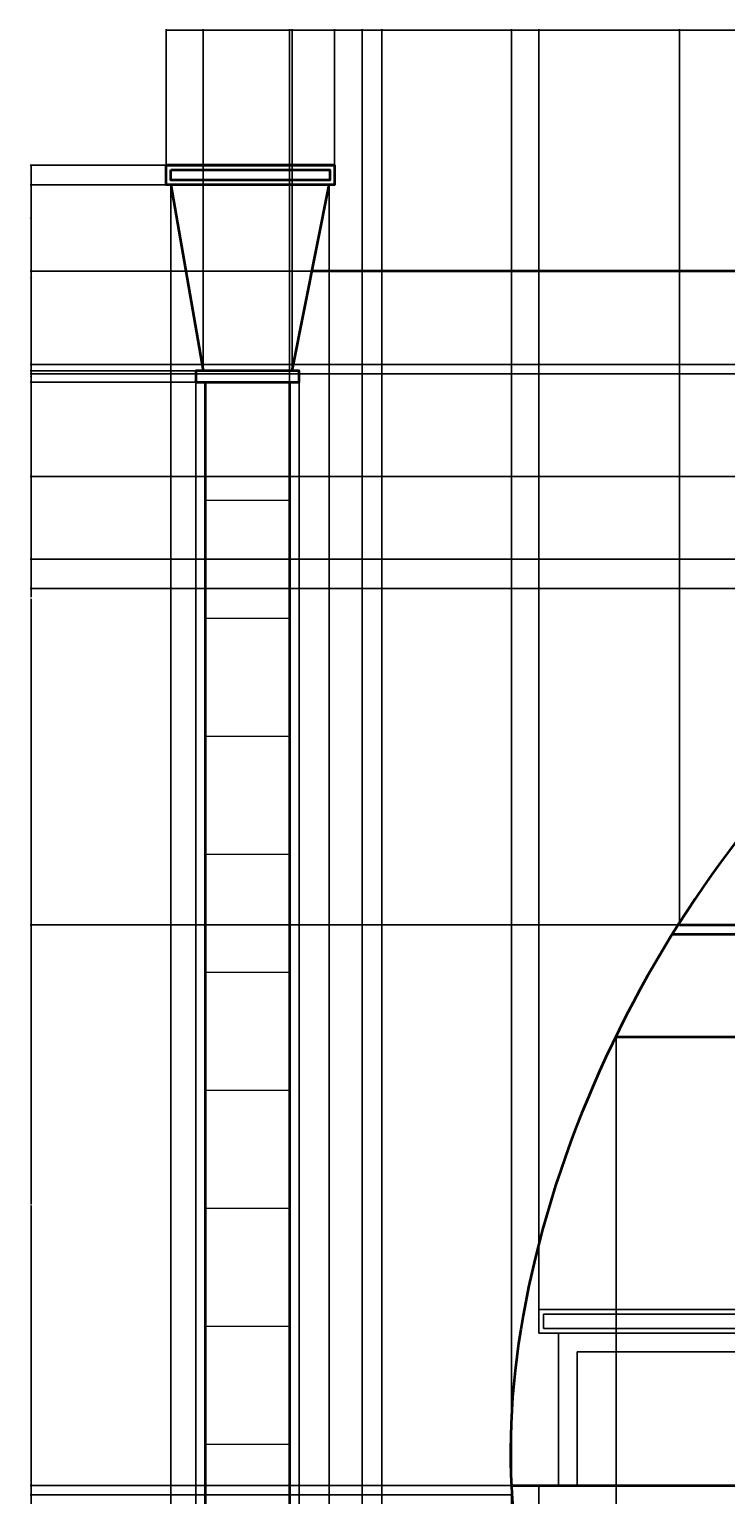
# Model space of a CAD drawing. Units: inches. Extents: x -19 to 408, y -26 to 603.
# Tile 5 of 7: x -19 to 130, y 289 to 603. Entities that reach past the tile are written whole.
import ezdxf

# ---------------------------------------------------------------- set-up
doc = ezdxf.new("R2010")
doc.units = ezdxf.units.IN
doc.header["$MEASUREMENT"] = 0
for name, color, linetype, lineweight in [('A-ANNO-DIMS', 2, 'Continuous', 18), ('A-ELEV', 7, 'Continuous', 35), ('A-GLAZ', 4, 'Continuous', 25), ('A-WALL-PATT', 8, 'Continuous', 13)]:
    doc.layers.add(name, color=color, linetype=linetype, lineweight=lineweight)
doc.styles.get("Standard").update_dxf_attribs({"font": 'arial.ttf'})
doc.dimstyles.get("Standard").update_dxf_attribs({"dimtxt": 0.18, "dimasz": 0.18, "dimexe": 0.18, "dimexo": 0.0625, "dimgap": 0.09, "dimtad": 0, "dimtih": 1, "dimtoh": 1, "dimdec": 4, "dimzin": 0, "dimdsep": 46, "dimtxsty": 'Standard', "dimcen": 0.09, "dimadec": 0, "dimazin": 0, "dimtfac": 1, "dimtdec": 4, "dimtofl": 0, "dimtmove": 0, "dimatfit": 3, "dimfxl": 1, "dimtolj": 1, "dimtzin": 0, "dimarcsym": 0})

# ---------------------------------------------------------------- blocks, each defined once
blk = doc.blocks.new('WIN-1200')
for points in [[(0, 32.56), (59.66, 32.56), (59.66, 37.64), (0, 37.64)], [(1, 33.56), (58.66, 33.56), (58.66, 36.64), (1, 36.64)]]:
    blk.add_lwpolyline(points, close=True)
for points in [[(4.17, 0), (4.17, 32.56), (55.99, 32.56), (55.99, 0)], [(8.17, 0), (8.17, 28.56), (51.99, 28.56), (51.99, 0)]]:
    blk.add_lwpolyline(points)
blk = doc.blocks.new('*D4')
at = {"layer": 'A-ANNO-DIMS', "color": 0, "lineweight": -2, "transparency": 16777216}
for p, q in [((89.99, 291.08), (89.99, 282.02)), ((149.65, 291.08), (149.65, 282.02)), ((90.17, 282.2), (118.7, 282.2)), ((149.47, 282.2), (120.94, 282.2))]:
    blk.add_line(p, q, dxfattribs=at)
at = {"layer": 'A-ANNO-DIMS', "color": 0, "transparency": 16777216}
for points in [[(90.17, 282.23), (90.17, 282.17), (89.99, 282.2)], [(149.47, 282.23), (149.47, 282.17), (149.65, 282.2)]]:
    blk.add_solid(points, dxfattribs=at)
at = {"layer": 'Defpoints', "color": 0, "transparency": 16777216}
for p in [(89.99, 291.15), (149.65, 291.15), (149.65, 282.2)]:
    blk.add_point(p, dxfattribs=at)
at = {"layer": 'A-ANNO-DIMS', "color": 0, "transparency": 16777216, "insert": (119.82, 282.2), "char_height": 0.18, "attachment_point": 5}
blk.add_mtext('\\A1;WINDOW 60 TYP.', dxfattribs=at)
blk = doc.blocks.new('*D15')
at = {"layer": 'A-ANNO-DIMS', "color": 0, "lineweight": -2, "transparency": 16777216}
for p, q in [((10.2, 573.88), (10.2, 602.9)), ((10.38, 602.72), (110.85, 602.72)), ((212.25, 602.72), (111.78, 602.72)), ((212.43, 551.17), (212.43, 602.9))]:
    blk.add_line(p, q, dxfattribs=at)
at = {"layer": 'A-ANNO-DIMS', "color": 0, "transparency": 16777216}
for points in [[(10.38, 602.75), (10.38, 602.69), (10.2, 602.72)], [(212.25, 602.75), (212.25, 602.69), (212.43, 602.72)]]:
    blk.add_solid(points, dxfattribs=at)
at = {"layer": 'Defpoints', "color": 0, "transparency": 16777216}
for p in [(212.43, 602.72), (10.2, 573.82), (212.43, 551.1)]:
    blk.add_point(p, dxfattribs=at)
at = {"layer": 'A-ANNO-DIMS', "color": 0, "transparency": 16777216, "insert": (111.32, 602.72), "char_height": 0.18, "attachment_point": 5}
blk.add_mtext('\\A1;202.23', dxfattribs=at)
blk = doc.blocks.new('*D19')
at = {"layer": 'A-ANNO-DIMS', "color": 0, "lineweight": -2, "transparency": 16777216}
for p, q in [((84.02, 291.15), (-18.88, 291.15)), ((-18.7, 290.97), (-18.7, 255.33)), ((-18.7, 219.33), (-18.7, 254.97)), ((36.51, 219.15), (-18.88, 219.15))]:
    blk.add_line(p, q, dxfattribs=at)
at = {"layer": 'A-ANNO-DIMS', "color": 0, "transparency": 16777216}
for points in [[(-18.73, 290.97), (-18.67, 290.97), (-18.7, 291.15)], [(-18.73, 219.33), (-18.67, 219.33), (-18.7, 219.15)]]:
    blk.add_solid(points, dxfattribs=at)
at = {"layer": 'Defpoints', "color": 0, "transparency": 16777216}
for p in [(-18.7, 291.15), (84.08, 291.15), (36.57, 219.15)]:
    blk.add_point(p, dxfattribs=at)
at = {"layer": 'A-ANNO-DIMS', "color": 0, "transparency": 16777216, "insert": (-18.7, 255.15), "char_height": 0.18, "attachment_point": 5}
blk.add_mtext('\\A1;72', dxfattribs=at)
blk = doc.blocks.new('*D20')
at = {"layer": 'A-ANNO-DIMS', "color": 0, "lineweight": -2, "transparency": 16777216}
for p, q in [((185.46, 411.15), (-18.88, 411.15)), ((-18.7, 410.97), (-18.7, 351.33)), ((-18.7, 291.33), (-18.7, 350.97)), ((84.02, 291.15), (-18.88, 291.15))]:
    blk.add_line(p, q, dxfattribs=at)
at = {"layer": 'A-ANNO-DIMS', "color": 0, "transparency": 16777216}
for points in [[(-18.73, 410.97), (-18.67, 410.97), (-18.7, 411.15)], [(-18.73, 291.33), (-18.67, 291.33), (-18.7, 291.15)]]:
    blk.add_solid(points, dxfattribs=at)
at = {"layer": 'Defpoints', "color": 0, "transparency": 16777216}
for p in [(-18.7, 411.15), (185.52, 411.15), (84.08, 291.15)]:
    blk.add_point(p, dxfattribs=at)
at = {"layer": 'A-ANNO-DIMS', "color": 0, "transparency": 16777216, "insert": (-18.7, 351.15), "char_height": 0.18, "attachment_point": 5}
blk.add_mtext('\\A1;120', dxfattribs=at)
blk = doc.blocks.new('*D21')
at = {"layer": 'A-ANNO-DIMS', "color": 0, "lineweight": -2, "transparency": 16777216}
for p, q in [((212.37, 551.1), (-18.88, 551.1)), ((-18.7, 550.92), (-18.7, 481.31)), ((-18.7, 411.33), (-18.7, 480.94)), ((185.46, 411.15), (-18.88, 411.15))]:
    blk.add_line(p, q, dxfattribs=at)
at = {"layer": 'A-ANNO-DIMS', "color": 0, "transparency": 16777216}
for points in [[(-18.73, 550.92), (-18.67, 550.92), (-18.7, 551.1)], [(-18.73, 411.33), (-18.67, 411.33), (-18.7, 411.15)]]:
    blk.add_solid(points, dxfattribs=at)
at = {"layer": 'Defpoints', "color": 0, "transparency": 16777216}
for p in [(-18.7, 551.1), (212.43, 551.1), (185.52, 411.15)]:
    blk.add_point(p, dxfattribs=at)
at = {"layer": 'A-ANNO-DIMS', "color": 0, "transparency": 16777216, "insert": (-18.7, 481.13), "char_height": 0.18, "attachment_point": 5}
blk.add_mtext('\\A1;139.96', dxfattribs=at)
blk = doc.blocks.new('*D22')
at = {"layer": 'A-ANNO-DIMS', "color": 0, "lineweight": -2, "transparency": 16777216}
for p, q in [((10.14, 573.82), (-18.88, 573.82)), ((-18.7, 573.64), (-18.7, 562.64)), ((-18.7, 551.28), (-18.7, 562.28)), ((212.37, 551.1), (-18.88, 551.1))]:
    blk.add_line(p, q, dxfattribs=at)
at = {"layer": 'A-ANNO-DIMS', "color": 0, "transparency": 16777216}
for points in [[(-18.73, 573.64), (-18.67, 573.64), (-18.7, 573.82)], [(-18.73, 551.28), (-18.67, 551.28), (-18.7, 551.1)]]:
    blk.add_solid(points, dxfattribs=at)
at = {"layer": 'Defpoints', "color": 0, "transparency": 16777216}
for p in [(-18.7, 573.82), (10.2, 573.82), (212.43, 551.1)]:
    blk.add_point(p, dxfattribs=at)
at = {"layer": 'A-ANNO-DIMS', "color": 0, "transparency": 16777216, "insert": (-18.7, 562.46), "char_height": 0.18, "attachment_point": 5}
blk.add_mtext('\\A1;22.714', dxfattribs=at)
blk = doc.blocks.new('*D28')
at = {"layer": 'A-ANNO-DIMS', "color": 0, "lineweight": -2, "transparency": 16777216}
for p, q in [((36.57, 300.05), (36.57, 602.9)), ((36.75, 602.72), (59.94, 602.72)), ((83.9, 602.72), (60.7, 602.72)), ((84.08, 291.21), (84.08, 602.9))]:
    blk.add_line(p, q, dxfattribs=at)
at = {"layer": 'A-ANNO-DIMS', "color": 0, "transparency": 16777216}
for points in [[(36.75, 602.75), (36.75, 602.69), (36.57, 602.72)], [(83.9, 602.75), (83.9, 602.69), (84.08, 602.72)]]:
    blk.add_solid(points, dxfattribs=at)
at = {"layer": 'Defpoints', "color": 0, "transparency": 16777216}
for p in [(84.08, 602.72), (36.57, 299.99), (84.08, 291.15)]:
    blk.add_point(p, dxfattribs=at)
at = {"layer": 'A-ANNO-DIMS', "color": 0, "transparency": 16777216, "insert": (60.32, 602.72), "char_height": 0.18, "attachment_point": 5}
blk.add_mtext('\\A1;47.51', dxfattribs=at)
blk = doc.blocks.new('*D35')
at = {"layer": 'A-ANNO-DIMS', "color": 0, "lineweight": -2, "transparency": 16777216}
for p, q in [((36.57, 171.21), (36.57, 602.9)), ((36.75, 602.72), (43.91, 602.72)), ((51.97, 602.72), (44.82, 602.72)), ((52.15, 203.77), (52.15, 602.9))]:
    blk.add_line(p, q, dxfattribs=at)
at = {"layer": 'A-ANNO-DIMS', "color": 0, "transparency": 16777216}
for points in [[(36.75, 602.75), (36.75, 602.69), (36.57, 602.72)], [(51.97, 602.75), (51.97, 602.69), (52.15, 602.72)]]:
    blk.add_solid(points, dxfattribs=at)
at = {"layer": 'Defpoints', "color": 0, "transparency": 16777216}
for p in [(52.15, 602.72), (52.15, 203.7), (36.57, 171.15)]:
    blk.add_point(p, dxfattribs=at)
at = {"layer": 'A-ANNO-DIMS', "color": 0, "transparency": 16777216, "insert": (44.36, 602.72), "char_height": 0.18, "attachment_point": 5}
blk.add_mtext('\\A1;15.582', dxfattribs=at)
blk = doc.blocks.new('*D36')
at = {"layer": 'A-ANNO-DIMS', "color": 0, "lineweight": -2, "transparency": 16777216}
for p, q in [((52.15, 203.77), (52.15, 602.9)), ((52.33, 602.72), (96.69, 602.72)), ((141.84, 602.72), (97.48, 602.72)), ((142.02, 171.21), (142.02, 602.9))]:
    blk.add_line(p, q, dxfattribs=at)
at = {"layer": 'A-ANNO-DIMS', "color": 0, "transparency": 16777216}
for points in [[(52.33, 602.75), (52.33, 602.69), (52.15, 602.72)], [(141.84, 602.75), (141.84, 602.69), (142.02, 602.72)]]:
    blk.add_solid(points, dxfattribs=at)
at = {"layer": 'Defpoints', "color": 0, "transparency": 16777216}
for p in [(142.02, 602.72), (52.15, 203.7), (142.02, 171.15)]:
    blk.add_point(p, dxfattribs=at)
at = {"layer": 'A-ANNO-DIMS', "color": 0, "transparency": 16777216, "insert": (97.09, 602.72), "char_height": 0.18, "attachment_point": 5}
blk.add_mtext('\\A1;89.87', dxfattribs=at)
blk = doc.blocks.new('*D45')
at = {"layer": 'A-ANNO-DIMS', "color": 0, "lineweight": -2, "transparency": 16777216}
for p, q in [((36.57, 219.21), (36.57, 602.9)), ((36.75, 602.72), (85.2, 602.72)), ((134.3, 602.72), (85.85, 602.72)), ((134.48, 220.21), (134.48, 602.9))]:
    blk.add_line(p, q, dxfattribs=at)
at = {"layer": 'A-ANNO-DIMS', "color": 0, "transparency": 16777216}
for points in [[(36.75, 602.75), (36.75, 602.69), (36.57, 602.72)], [(134.3, 602.75), (134.3, 602.69), (134.48, 602.72)]]:
    blk.add_solid(points, dxfattribs=at)
at = {"layer": 'Defpoints', "color": 0, "transparency": 16777216}
for p in [(134.48, 602.72), (134.48, 220.15), (36.57, 219.15)]:
    blk.add_point(p, dxfattribs=at)
at = {"layer": 'A-ANNO-DIMS', "color": 0, "transparency": 16777216, "insert": (85.52, 602.72), "char_height": 0.18, "attachment_point": 5}
blk.add_mtext('\\A1;97.9', dxfattribs=at)
blk = doc.blocks.new('*D47')
at = {"layer": 'A-ANNO-DIMS', "color": 0, "lineweight": -2, "transparency": 16777216}
for p, q in [((52.15, 203.77), (52.15, 602.9)), ((52.33, 602.72), (53.84, 602.72)), ((56.15, 602.72), (54.64, 602.72)), ((56.33, 203.77), (56.33, 602.9))]:
    blk.add_line(p, q, dxfattribs=at)
at = {"layer": 'A-ANNO-DIMS', "color": 0, "transparency": 16777216}
for points in [[(52.33, 602.75), (52.33, 602.69), (52.15, 602.72)], [(56.15, 602.75), (56.15, 602.69), (56.33, 602.72)]]:
    blk.add_solid(points, dxfattribs=at)
at = {"layer": 'Defpoints', "color": 0, "transparency": 16777216}
for p in [(56.33, 602.72), (52.15, 203.7), (56.33, 203.7)]:
    blk.add_point(p, dxfattribs=at)
at = {"layer": 'A-ANNO-DIMS', "color": 0, "transparency": 16777216, "insert": (54.24, 602.72), "char_height": 0.18, "attachment_point": 5}
blk.add_mtext('\\A1;4.173', dxfattribs=at)
blk = doc.blocks.new('*D60')
at = {"layer": 'A-ANNO-DIMS', "color": 0, "lineweight": -2, "transparency": 16777216}
for p, q in [((84.08, 291.08), (84.08, -25.93)), ((109.02, 267.08), (109.02, -25.93)), ((84.26, -25.75), (96.15, -25.75)), ((108.84, -25.75), (96.94, -25.75))]:
    blk.add_line(p, q, dxfattribs=at)
at = {"layer": 'A-ANNO-DIMS', "color": 0, "transparency": 16777216}
for points in [[(84.26, -25.72), (84.26, -25.78), (84.08, -25.75)], [(108.84, -25.72), (108.84, -25.78), (109.02, -25.75)]]:
    blk.add_solid(points, dxfattribs=at)
at = {"layer": 'Defpoints', "color": 0, "transparency": 16777216}
for p in [(84.08, 291.15), (109.02, 267.15), (109.02, -25.75)]:
    blk.add_point(p, dxfattribs=at)
at = {"layer": 'A-ANNO-DIMS', "color": 0, "transparency": 16777216, "insert": (96.55, -25.75), "char_height": 0.18, "attachment_point": 5}
blk.add_mtext('\\A1;24.94', dxfattribs=at)
blk = doc.blocks.new('*D66')
at = {"layer": 'A-ANNO-DIMS', "color": 0, "lineweight": -2, "transparency": 16777216}
for p, q in [((84.08, 291.21), (84.08, 602.9)), ((84.26, 602.72), (86.64, 602.72)), ((89.81, 602.72), (87.43, 602.72)), ((89.99, 323.77), (89.99, 602.9))]:
    blk.add_line(p, q, dxfattribs=at)
at = {"layer": 'A-ANNO-DIMS', "color": 0, "transparency": 16777216}
for points in [[(84.26, 602.75), (84.26, 602.69), (84.08, 602.72)], [(89.81, 602.75), (89.81, 602.69), (89.99, 602.72)]]:
    blk.add_solid(points, dxfattribs=at)
at = {"layer": 'Defpoints', "color": 0, "transparency": 16777216}
for p in [(89.99, 602.72), (89.99, 323.7), (84.08, 291.15)]:
    blk.add_point(p, dxfattribs=at)
at = {"layer": 'A-ANNO-DIMS', "color": 0, "transparency": 16777216, "insert": (87.03, 602.72), "char_height": 0.18, "attachment_point": 5}
blk.add_mtext('\\A1;5.912', dxfattribs=at)
blk = doc.blocks.new('*D68')
at = {"layer": 'A-ANNO-DIMS', "color": 0, "lineweight": -2, "transparency": 16777216}
for p, q in [((84.13, 289.15), (-18.88, 289.15)), ((-18.7, 288.97), (-18.7, 278.33)), ((-18.7, 267.33), (-18.7, 277.97)), ((87.66, 267.15), (-18.88, 267.15))]:
    blk.add_line(p, q, dxfattribs=at)
at = {"layer": 'A-ANNO-DIMS', "color": 0, "transparency": 16777216}
for points in [[(-18.73, 288.97), (-18.67, 288.97), (-18.7, 289.15)], [(-18.73, 267.33), (-18.67, 267.33), (-18.7, 267.15)]]:
    blk.add_solid(points, dxfattribs=at)
at = {"layer": 'Defpoints', "color": 0, "transparency": 16777216}
for p in [(-18.7, 289.15), (84.19, 289.15), (87.72, 267.15)]:
    blk.add_point(p, dxfattribs=at)
at = {"layer": 'A-ANNO-DIMS', "color": 0, "transparency": 16777216, "insert": (-18.7, 278.15), "char_height": 0.18, "attachment_point": 5}
blk.add_mtext('\\A1;22', dxfattribs=at)
blk = doc.blocks.new('*D69')
at = {"layer": 'A-ANNO-DIMS', "color": 0, "lineweight": -2, "transparency": 16777216}
for p, q in [((84.02, 291.15), (-18.88, 291.15)), ((84.13, 289.15), (-18.88, 289.15)), ((-18.7, 290.97), (-18.7, 290.33)), ((-18.7, 289.33), (-18.7, 289.97))]:
    blk.add_line(p, q, dxfattribs=at)
at = {"layer": 'A-ANNO-DIMS', "color": 0, "transparency": 16777216}
for points in [[(-18.73, 290.97), (-18.67, 290.97), (-18.7, 291.15)], [(-18.73, 289.33), (-18.67, 289.33), (-18.7, 289.15)]]:
    blk.add_solid(points, dxfattribs=at)
at = {"layer": 'Defpoints', "color": 0, "transparency": 16777216}
for p in [(-18.7, 291.15), (84.08, 291.15), (84.19, 289.15)]:
    blk.add_point(p, dxfattribs=at)
at = {"layer": 'A-ANNO-DIMS', "color": 0, "transparency": 16777216, "insert": (-18.7, 290.15), "char_height": 0.18, "attachment_point": 5}
blk.add_mtext('\\A1;2', dxfattribs=at)
blk = doc.blocks.new('*D79')
at = {"layer": 'A-ANNO-DIMS', "color": 0, "lineweight": -2, "transparency": 16777216}
for p, q in [((212.37, 489.45), (-18.88, 489.45)), ((-18.7, 489.27), (-18.7, 486.48)), ((-18.7, 483.33), (-18.7, 486.12)), ((212.37, 483.15), (-18.88, 483.15))]:
    blk.add_line(p, q, dxfattribs=at)
at = {"layer": 'A-ANNO-DIMS', "color": 0, "transparency": 16777216}
for points in [[(-18.73, 489.27), (-18.67, 489.27), (-18.7, 489.45)], [(-18.73, 483.33), (-18.67, 483.33), (-18.7, 483.15)]]:
    blk.add_solid(points, dxfattribs=at)
at = {"layer": 'Defpoints', "color": 0, "transparency": 16777216}
for p in [(-18.7, 489.45), (212.43, 489.45), (212.43, 483.15)]:
    blk.add_point(p, dxfattribs=at)
at = {"layer": 'A-ANNO-DIMS', "color": 0, "transparency": 16777216, "insert": (-18.7, 486.3), "char_height": 0.18, "attachment_point": 5}
blk.add_mtext('\\A1;6.3', dxfattribs=at)
blk = doc.blocks.new('*D80')
at = {"layer": 'A-ANNO-DIMS', "color": 0, "lineweight": -2, "transparency": 16777216}
for p, q in [((212.37, 507.15), (-18.88, 507.15)), ((-18.7, 506.97), (-18.7, 495.33)), ((-18.7, 483.33), (-18.7, 494.97)), ((212.37, 483.15), (-18.88, 483.15))]:
    blk.add_line(p, q, dxfattribs=at)
at = {"layer": 'A-ANNO-DIMS', "color": 0, "transparency": 16777216}
for points in [[(-18.73, 506.97), (-18.67, 506.97), (-18.7, 507.15)], [(-18.73, 483.33), (-18.67, 483.33), (-18.7, 483.15)]]:
    blk.add_solid(points, dxfattribs=at)
at = {"layer": 'Defpoints', "color": 0, "transparency": 16777216}
for p in [(-18.7, 507.15), (212.43, 507.15), (212.43, 483.15)]:
    blk.add_point(p, dxfattribs=at)
at = {"layer": 'A-ANNO-DIMS', "color": 0, "transparency": 16777216, "insert": (-18.7, 495.15), "char_height": 0.18, "attachment_point": 5}
blk.add_mtext('\\A1;24', dxfattribs=at)
blk = doc.blocks.new('*D81')
at = {"layer": 'A-ANNO-DIMS', "color": 0, "lineweight": -2, "transparency": 16777216}
for p, q in [((212.37, 531.15), (-18.88, 531.15)), ((-18.7, 530.97), (-18.7, 530.33)), ((212.37, 529.15), (-18.88, 529.15)), ((-18.7, 529.33), (-18.7, 529.97))]:
    blk.add_line(p, q, dxfattribs=at)
at = {"layer": 'A-ANNO-DIMS', "color": 0, "transparency": 16777216}
for points in [[(-18.73, 530.97), (-18.67, 530.97), (-18.7, 531.15)], [(-18.73, 529.33), (-18.67, 529.33), (-18.7, 529.15)]]:
    blk.add_solid(points, dxfattribs=at)
at = {"layer": 'Defpoints', "color": 0, "transparency": 16777216}
for p in [(-18.7, 531.15), (212.43, 531.15), (212.43, 529.15)]:
    blk.add_point(p, dxfattribs=at)
at = {"layer": 'A-ANNO-DIMS', "color": 0, "transparency": 16777216, "insert": (-18.7, 530.15), "char_height": 0.18, "attachment_point": 5}
blk.add_mtext('\\A1;2', dxfattribs=at)
blk = doc.blocks.new('*D97')
at = {"layer": 'A-ANNO-DIMS', "color": 0, "lineweight": -2, "transparency": 16777216}
for p, q in [((10.2, 573.88), (10.2, 602.9)), ((10.38, 602.72), (27.77, 602.72)), ((46.08, 602.72), (28.69, 602.72)), ((46.26, 573.88), (46.26, 602.9))]:
    blk.add_line(p, q, dxfattribs=at)
at = {"layer": 'A-ANNO-DIMS', "color": 0, "transparency": 16777216}
for points in [[(10.38, 602.75), (10.38, 602.69), (10.2, 602.72)], [(46.08, 602.75), (46.08, 602.69), (46.26, 602.72)]]:
    blk.add_solid(points, dxfattribs=at)
at = {"layer": 'Defpoints', "color": 0, "transparency": 16777216}
for p in [(46.26, 602.72), (10.2, 573.82), (46.26, 573.82)]:
    blk.add_point(p, dxfattribs=at)
at = {"layer": 'A-ANNO-DIMS', "color": 0, "transparency": 16777216, "insert": (28.23, 602.72), "char_height": 0.18, "attachment_point": 5}
blk.add_mtext('\\A1;36.054', dxfattribs=at)
blk = doc.blocks.new('*D98')
at = {"layer": 'A-ANNO-DIMS', "color": 0, "lineweight": -2, "transparency": 16777216}
for p, q in [((10.14, 573.82), (-18.88, 573.82)), ((-18.7, 573.64), (-18.7, 571.89)), ((-18.7, 569.79), (-18.7, 571.53)), ((10.14, 569.61), (-18.88, 569.61))]:
    blk.add_line(p, q, dxfattribs=at)
at = {"layer": 'A-ANNO-DIMS', "color": 0, "transparency": 16777216}
for points in [[(-18.73, 573.64), (-18.67, 573.64), (-18.7, 573.82)], [(-18.73, 569.79), (-18.67, 569.79), (-18.7, 569.61)]]:
    blk.add_solid(points, dxfattribs=at)
at = {"layer": 'Defpoints', "color": 0, "transparency": 16777216}
for p in [(-18.7, 573.82), (10.2, 573.82), (10.2, 569.61)]:
    blk.add_point(p, dxfattribs=at)
at = {"layer": 'A-ANNO-DIMS', "color": 0, "transparency": 16777216, "insert": (-18.7, 571.71), "char_height": 0.18, "attachment_point": 5}
blk.add_mtext('\\A1;4.213', dxfattribs=at)
blk = doc.blocks.new('*D99')
at = {"layer": 'A-ANNO-DIMS', "color": 0, "lineweight": -2, "transparency": 16777216}
for p, q in [((11.24, 569.54), (11.24, -25.93)), ((45.11, 569.54), (45.11, -25.93)), ((11.42, -25.75), (27.71, -25.75)), ((44.93, -25.75), (28.64, -25.75))]:
    blk.add_line(p, q, dxfattribs=at)
at = {"layer": 'A-ANNO-DIMS', "color": 0, "transparency": 16777216}
for points in [[(11.42, -25.72), (11.42, -25.78), (11.24, -25.75)], [(44.93, -25.72), (44.93, -25.78), (45.11, -25.75)]]:
    blk.add_solid(points, dxfattribs=at)
at = {"layer": 'Defpoints', "color": 0, "transparency": 16777216}
for p in [(11.24, 569.61), (45.11, 569.61), (45.11, -25.75)]:
    blk.add_point(p, dxfattribs=at)
at = {"layer": 'A-ANNO-DIMS', "color": 0, "transparency": 16777216, "insert": (28.17, -25.75), "char_height": 0.18, "attachment_point": 5}
blk.add_mtext('\\A1;33.876', dxfattribs=at)
blk = doc.blocks.new('*D100')
at = {"layer": 'A-ANNO-DIMS', "color": 0, "lineweight": -2, "transparency": 16777216}
for p, q in [((18.16, 529.8), (18.16, 602.9)), ((18.34, 602.72), (27.27, 602.72)), ((36.97, 602.72), (28.04, 602.72)), ((37.15, 529.8), (37.15, 602.9))]:
    blk.add_line(p, q, dxfattribs=at)
at = {"layer": 'A-ANNO-DIMS', "color": 0, "transparency": 16777216}
for points in [[(18.34, 602.75), (18.34, 602.69), (18.16, 602.72)], [(36.97, 602.75), (36.97, 602.69), (37.15, 602.72)]]:
    blk.add_solid(points, dxfattribs=at)
at = {"layer": 'Defpoints', "color": 0, "transparency": 16777216}
for p in [(37.15, 602.72), (18.16, 529.74), (37.15, 529.74)]:
    blk.add_point(p, dxfattribs=at)
at = {"layer": 'A-ANNO-DIMS', "color": 0, "transparency": 16777216, "insert": (27.65, 602.72), "char_height": 0.18, "attachment_point": 5}
blk.add_mtext('\\A1;18.99', dxfattribs=at)
blk = doc.blocks.new('*D101')
at = {"layer": 'A-ANNO-DIMS', "color": 0, "lineweight": -2, "transparency": 16777216}
for p, q in [((16.55, 527.3), (16.55, -25.93)), ((38.69, 527.3), (38.69, -25.93)), ((16.73, -25.75), (27.16, -25.75)), ((38.51, -25.75), (28.09, -25.75))]:
    blk.add_line(p, q, dxfattribs=at)
at = {"layer": 'A-ANNO-DIMS', "color": 0, "transparency": 16777216}
for points in [[(16.73, -25.72), (16.73, -25.78), (16.55, -25.75)], [(38.51, -25.72), (38.51, -25.78), (38.69, -25.75)]]:
    blk.add_solid(points, dxfattribs=at)
at = {"layer": 'Defpoints', "color": 0, "transparency": 16777216}
for p in [(16.55, 527.36), (38.69, 527.36), (38.69, -25.75)]:
    blk.add_point(p, dxfattribs=at)
at = {"layer": 'A-ANNO-DIMS', "color": 0, "transparency": 16777216, "insert": (27.62, -25.75), "char_height": 0.18, "attachment_point": 5}
blk.add_mtext('\\A1;22.143', dxfattribs=at)
blk = doc.blocks.new('*D102')
at = {"layer": 'A-ANNO-DIMS', "color": 0, "lineweight": -2, "transparency": 16777216}
for p, q in [((16.49, 529.74), (-18.88, 529.74)), ((16.49, 527.36), (-18.88, 527.36)), ((-18.7, 529.56), (-18.7, 528.73)), ((-18.7, 527.54), (-18.7, 528.37))]:
    blk.add_line(p, q, dxfattribs=at)
at = {"layer": 'A-ANNO-DIMS', "color": 0, "transparency": 16777216}
for points in [[(-18.73, 529.56), (-18.67, 529.56), (-18.7, 529.74)], [(-18.73, 527.54), (-18.67, 527.54), (-18.7, 527.36)]]:
    blk.add_solid(points, dxfattribs=at)
at = {"layer": 'Defpoints', "color": 0, "transparency": 16777216}
for p in [(-18.7, 529.74), (16.55, 529.74), (16.55, 527.36)]:
    blk.add_point(p, dxfattribs=at)
at = {"layer": 'A-ANNO-DIMS', "color": 0, "transparency": 16777216, "insert": (-18.7, 528.55), "char_height": 0.18, "attachment_point": 5}
blk.add_mtext('\\A1;2.38', dxfattribs=at)
blk = doc.blocks.new('*D103')
at = {"layer": 'A-ANNO-DIMS', "color": 0, "lineweight": -2, "transparency": 16777216}
for p, q in [((11.17, 569.61), (-18.88, 569.61)), ((-18.7, 569.43), (-18.7, 549.86)), ((-18.7, 529.92), (-18.7, 549.49)), ((18.09, 529.74), (-18.88, 529.74))]:
    blk.add_line(p, q, dxfattribs=at)
at = {"layer": 'A-ANNO-DIMS', "color": 0, "transparency": 16777216}
for points in [[(-18.73, 569.43), (-18.67, 569.43), (-18.7, 569.61)], [(-18.73, 529.92), (-18.67, 529.92), (-18.7, 529.74)]]:
    blk.add_solid(points, dxfattribs=at)
at = {"layer": 'Defpoints', "color": 0, "transparency": 16777216}
for p in [(-18.7, 569.61), (11.24, 569.61), (18.16, 529.74)]:
    blk.add_point(p, dxfattribs=at)
at = {"layer": 'A-ANNO-DIMS', "color": 0, "transparency": 16777216, "insert": (-18.7, 549.67), "char_height": 0.18, "attachment_point": 5}
blk.add_mtext('\\A1;39.86', dxfattribs=at)
blk = doc.blocks.new('*D104')
at = {"layer": 'A-ANNO-DIMS', "color": 0, "lineweight": -2, "transparency": 16777216}
for p, q in [((16.55, 527.3), (16.55, -25.93)), ((18.57, 527.3), (18.57, -25.93)), ((16.73, -25.75), (17.24, -25.75)), ((18.39, -25.75), (17.88, -25.75))]:
    blk.add_line(p, q, dxfattribs=at)
at = {"layer": 'A-ANNO-DIMS', "color": 0, "transparency": 16777216}
for points in [[(16.73, -25.72), (16.73, -25.78), (16.55, -25.75)], [(18.39, -25.72), (18.39, -25.78), (18.57, -25.75)]]:
    blk.add_solid(points, dxfattribs=at)
at = {"layer": 'Defpoints', "color": 0, "transparency": 16777216}
for p in [(16.55, 527.36), (18.57, 527.36), (18.57, -25.75)]:
    blk.add_point(p, dxfattribs=at)
at = {"layer": 'A-ANNO-DIMS', "color": 0, "transparency": 16777216, "insert": (17.56, -25.75), "char_height": 0.18, "attachment_point": 5}
blk.add_mtext('\\A1;2.02', dxfattribs=at)
blk = doc.blocks.new('*D105')
at = {"layer": 'A-ANNO-DIMS', "color": 0, "lineweight": -2, "transparency": 16777216}
for p, q in [((120.05, 411.21), (120.05, 602.9)), ((120.23, 602.72), (152.39, 602.72)), ((185.34, 602.72), (153.18, 602.72)), ((185.52, 411.21), (185.52, 602.9))]:
    blk.add_line(p, q, dxfattribs=at)
at = {"layer": 'A-ANNO-DIMS', "color": 0, "transparency": 16777216}
for points in [[(120.23, 602.75), (120.23, 602.69), (120.05, 602.72)], [(185.34, 602.75), (185.34, 602.69), (185.52, 602.72)]]:
    blk.add_solid(points, dxfattribs=at)
at = {"layer": 'Defpoints', "color": 0, "transparency": 16777216}
for p in [(120.05, 602.72), (120.05, 411.15), (185.52, 411.15)]:
    blk.add_point(p, dxfattribs=at)
at = {"layer": 'A-ANNO-DIMS', "color": 0, "transparency": 16777216, "insert": (152.79, 602.72), "char_height": 0.18, "attachment_point": 5}
blk.add_mtext('\\A1;65.47', dxfattribs=at)
blk = doc.blocks.new('*D106')
at = {"layer": 'A-ANNO-DIMS', "color": 0, "lineweight": -2, "transparency": 16777216}
for p, q in [((106.54, 387.08), (106.54, -25.93)), ((185.52, 387.08), (185.52, -25.93)), ((106.72, -25.75), (145.64, -25.75)), ((185.34, -25.75), (146.43, -25.75))]:
    blk.add_line(p, q, dxfattribs=at)
at = {"layer": 'A-ANNO-DIMS', "color": 0, "transparency": 16777216}
for points in [[(106.72, -25.72), (106.72, -25.78), (106.54, -25.75)], [(185.34, -25.72), (185.34, -25.78), (185.52, -25.75)]]:
    blk.add_solid(points, dxfattribs=at)
at = {"layer": 'Defpoints', "color": 0, "transparency": 16777216}
for p in [(106.54, 387.15), (185.52, 387.15), (106.54, -25.75)]:
    blk.add_point(p, dxfattribs=at)
at = {"layer": 'A-ANNO-DIMS', "color": 0, "transparency": 16777216, "insert": (146.03, -25.75), "char_height": 0.18, "attachment_point": 5}
blk.add_mtext('\\A1;78.98', dxfattribs=at)

msp = doc.modelspace()

# ---------------------------------------------------------------- linework, layer by layer
at = {"layer": 'A-ELEV'}
for p, q in [((212.4303, 551.1043), (41.4148, 551.1043)), ((18.5712, 527.3578), (18.5712, 123.1472)), ((36.5712, 527.3578), (36.5712, 3.1472)), ((120.0489, 411.1472), (360.5712, 411.1472)), ((118.7171, 409.1472), (185.5212, 409.1472)), ((106.5444, 387.1472), (185.5212, 387.1472)), ((84.0785, 291.1472), (300.5581, 291.1472))]:
    msp.add_line(p, q, dxfattribs=at)
for points in [[(10.202, 573.8184), (46.256, 573.8184), (46.256, 569.605), (10.202, 569.605)], [(11.202, 572.8184), (45.256, 572.8184), (45.256, 570.605), (11.202, 570.605)], [(16.5486, 527.3578), (38.6921, 527.3578), (38.6921, 529.7414), (16.5486, 529.7414)]]:
    msp.add_lwpolyline(points, close=True, dxfattribs=at)
for points in [[(45.9539, 573.8184), (10.5041, 573.8184)], [(11.2357, 569.605), (18.1573, 529.7414)], [(37.1458, 529.7414), (45.1119, 569.605)], [(18.5712, 527.3578), (18.5712, 527.3578), (36.6694, 527.3578)]]:
    msp.add_lwpolyline(points, dxfattribs=at)
msp.add_ellipse((188.4962, 355.8525), major_axis=(71.2607, 129.8447), ratio=0.58959924, start_param=6.80188927, end_param=9.63162337, dxfattribs=at)
at = {"layer": 'A-WALL-PATT'}
for p, q in [((18.5712, 527.3578), (36.5712, 527.3578)), ((18.5712, 502.0946), (36.5712, 502.0946)), ((18.5712, 476.8314), (36.5712, 476.8314)), ((18.5712, 451.5683), (36.5712, 451.5683)), ((18.5712, 426.3051), (36.5712, 426.3051)), ((18.5712, 401.042), (36.5712, 401.042)), ((18.5712, 375.7788), (36.5712, 375.7788)), ((18.5712, 350.5157), (36.5712, 350.5157)), ((18.5712, 325.2525), (36.5712, 325.2525)), ((18.5712, 299.9893), (36.5712, 299.9893))]:
    msp.add_line(p, q, dxfattribs=at)

# ---------------------------------------------------------------- block references
at = {"layer": 'A-GLAZ'}
msp.add_blockref('WIN-1200', (89.9903, 291.147), dxfattribs=at)

# ---------------------------------------------------------------- dimensions: what is measured, and where the dimension line sits
at = {"layer": 'A-ANNO-DIMS'}
for base, p1, p2, override, picture, middle in [((212.4303, 602.7184), (10.202, 573.8184), (212.4303, 551.1043), {"dimdec": 2, "dimlfac": 1, "dimrnd": 0, "dimzin": 0, "dimdsep": 46, "dimlunit": 2}, '*D15', (111.3162, 602.7184)), ((46.256, 602.7184), (10.202, 573.8184), (46.256, 573.8184), {"dimdec": 3, "dimlfac": 1, "dimrnd": 0, "dimzin": 0, "dimdsep": 46, "dimlunit": 2}, '*D97', (28.229, 602.7184)), ((37.1458, 602.7184), (18.1573, 529.7414), (37.1458, 529.7414), {"dimdec": 2, "dimlfac": 1, "dimrnd": 0, "dimzin": 0, "dimdsep": 46, "dimlunit": 2}, '*D100', (27.6515, 602.7184)), ((84.0785, 602.7184), (36.5712, 299.9893), (84.0785, 291.1472), {"dimdec": 2, "dimlfac": 1, "dimrnd": 0, "dimzin": 0, "dimdsep": 46, "dimlunit": 2}, '*D28', (60.3249, 602.7184)), ((52.1528, 602.7184), (36.5712, 171.1472), (52.1528, 203.704), {"dimdec": 3, "dimlfac": 1, "dimrnd": 0, "dimzin": 0, "dimdsep": 46, "dimlunit": 2}, '*D35', (44.362, 602.7184)), ((134.4772, 602.7184), (36.5712, 219.1472), (134.4772, 220.1467), {"dimdec": 1, "dimlfac": 1, "dimrnd": 0, "dimzin": 0, "dimdsep": 46, "dimlunit": 2}, '*D45', (85.5242, 602.7184)), ((142.0243, 602.7184), (52.1528, 203.704), (142.0243, 171.1472), {"dimdec": 2, "dimlfac": 1, "dimrnd": 0, "dimzin": 0, "dimdsep": 46, "dimlunit": 2}, '*D36', (97.0885, 602.7184)), ((56.3261, 602.7184), (52.1528, 203.704), (56.3261, 203.704), {"dimdec": 3, "dimlfac": 1, "dimrnd": 0, "dimzin": 0, "dimdsep": 46, "dimlunit": 2}, '*D47', (54.2394, 602.7184)), ((89.9901, 602.7184), (84.0785, 291.1472), (89.9901, 323.704), {"dimdec": 3, "dimlfac": 1, "dimrnd": 0, "dimzin": 0, "dimdsep": 46, "dimlunit": 2}, '*D66', (87.0343, 602.7184)), ((120.0489, 602.7184), (185.5212, 411.1472), (120.0489, 411.1472), {"dimdec": 2, "dimlfac": 1, "dimrnd": 0, "dimzin": 0, "dimdsep": 46, "dimlunit": 2}, '*D105', (152.7851, 602.7184)), ((45.1119, -25.7528), (11.2357, 569.605), (45.1119, 569.605), {"dimdec": 3, "dimlfac": 1, "dimrnd": 0, "dimzin": 0, "dimdsep": 46, "dimlunit": 2}, '*D99', (28.1738, -25.7528)), ((38.69205, -25.75277), (16.54859, 527.35776), (38.69205, 527.35776), {"dimdec": 3, "dimlfac": 1, "dimrnd": 0, "dimzin": 0, "dimdsep": 46, "dimlunit": 2}, '*D101', (27.62032, -25.75277)), ((18.5712, -25.7528), (16.5486, 527.3578), (18.5712, 527.3578), {"dimdec": 2, "dimlfac": 1, "dimrnd": 0, "dimzin": 0, "dimdsep": 46, "dimlunit": 2}, '*D104', (17.5599, -25.7528)), ((106.5444, -25.7528), (185.5212, 387.1472), (106.5444, 387.1472), {"dimdec": 2, "dimlfac": 1, "dimrnd": 0, "dimzin": 0, "dimdsep": 46, "dimlunit": 2}, '*D106', (146.0328, -25.7528)), ((109.0164, -25.7528), (84.0785, 291.1472), (109.0164, 267.1472), {"dimdec": 2, "dimlfac": 1, "dimrnd": 0, "dimzin": 0, "dimdsep": 46, "dimlunit": 2}, '*D60', (96.5475, -25.7528))]:
    dim = msp.add_linear_dim(base=base, p1=p1, p2=p2, dimstyle='Standard', override=override, dxfattribs=at)
    dim.commit()
    dim.dimension.update_dxf_attribs({"geometry": picture, "text_midpoint": middle})
for base, p1, p2, override, picture, middle in [((-18.698, 573.8184), (212.4303, 551.1043), (10.202, 573.8184), {"dimdec": 3, "dimlfac": 1, "dimrnd": 0, "dimzin": 0, "dimdsep": 46, "dimlunit": 2}, '*D22', (-18.698, 562.4614)), ((-18.698, 573.8184), (10.202, 569.605), (10.202, 573.8184), {"dimdec": 3, "dimlfac": 1, "dimrnd": 0, "dimzin": 0, "dimdsep": 46, "dimlunit": 2}, '*D98', (-18.698, 571.7117)), ((-18.698, 569.605), (18.1573, 529.7414), (11.2357, 569.605), {"dimdec": 2, "dimlfac": 1, "dimrnd": 0, "dimzin": 0, "dimdsep": 46, "dimlunit": 2}, '*D103', (-18.698, 549.6732)), ((-18.698, 551.1043), (185.5212, 411.1472), (212.4303, 551.1043), {"dimdec": 2, "dimlfac": 1, "dimrnd": 0, "dimzin": 0, "dimdsep": 46, "dimlunit": 2}, '*D21', (-18.698, 481.1258)), ((-18.698, 531.1472), (212.4303, 529.1472), (212.4303, 531.1472), {"dimdec": 0, "dimlfac": 1, "dimrnd": 0, "dimzin": 0, "dimdsep": 46, "dimlunit": 2}, '*D81', (-18.698, 530.1472)), ((-18.698, 529.7414), (16.5486, 527.3578), (16.5486, 529.7414), {"dimdec": 2, "dimlfac": 1, "dimrnd": 0, "dimzin": 0, "dimdsep": 46, "dimlunit": 2}, '*D102', (-18.698, 528.5496)), ((-18.698, 507.1472), (212.4303, 483.1472), (212.4303, 507.1472), {"dimdec": 0, "dimlfac": 1, "dimrnd": 0, "dimzin": 0, "dimdsep": 46, "dimlunit": 2}, '*D80', (-18.698, 495.1472)), ((-18.698, 489.4471), (212.4303, 483.1472), (212.4303, 489.4471), {"dimdec": 1, "dimlfac": 1, "dimrnd": 0, "dimzin": 0, "dimdsep": 46, "dimlunit": 2}, '*D79', (-18.698, 486.2971)), ((-18.698, 411.1472), (84.0785, 291.1472), (185.5212, 411.1472), {"dimdec": 0, "dimlfac": 1, "dimrnd": 0, "dimzin": 0, "dimdsep": 46, "dimlunit": 2}, '*D20', (-18.698, 351.1472)), ((-18.698, 291.1472), (36.5712, 219.1472), (84.0785, 291.1472), {"dimdec": 0, "dimlfac": 1, "dimrnd": 0, "dimzin": 0, "dimdsep": 46, "dimlunit": 2}, '*D19', (-18.698, 255.1472)), ((-18.698, 291.1472), (84.1933, 289.1472), (84.0785, 291.1472), {"dimdec": 0, "dimlfac": 1, "dimrnd": 0, "dimzin": 0, "dimdsep": 46, "dimlunit": 2}, '*D69', (-18.698, 290.1472)), ((-18.698, 289.1472), (87.7217, 267.1472), (84.1933, 289.1472), {"dimdec": 0, "dimlfac": 1, "dimrnd": 0, "dimzin": 0, "dimdsep": 46, "dimlunit": 2}, '*D68', (-18.698, 278.1472))]:
    dim = msp.add_linear_dim(base=base, p1=p1, p2=p2, angle=90, dimstyle='Standard', override=override, dxfattribs=at)
    dim.commit()
    dim.dimension.update_dxf_attribs({"geometry": picture, "text_midpoint": middle})
dim = msp.add_linear_dim(base=(149.6464, 282.1988), p1=(89.9901, 291.1472), p2=(149.6464, 291.1472), text='WINDOW <> TYP.', dimstyle='Standard', override={"dimdec": 0, "dimlfac": 1, "dimrnd": 0, "dimzin": 0, "dimdsep": 46, "dimlunit": 2}, dxfattribs=at)
dim.commit()
dim.dimension.update_dxf_attribs({"geometry": '*D4', "text_midpoint": (119.8182, 282.1988)})

doc.saveas('drawing.dxf')
